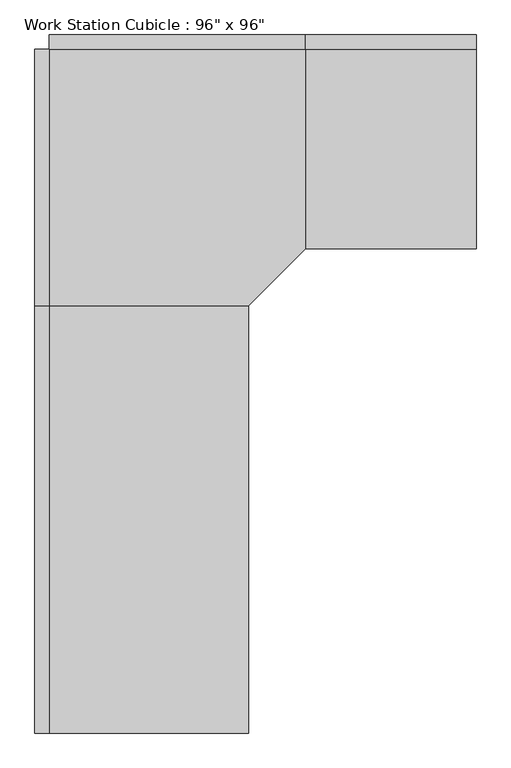
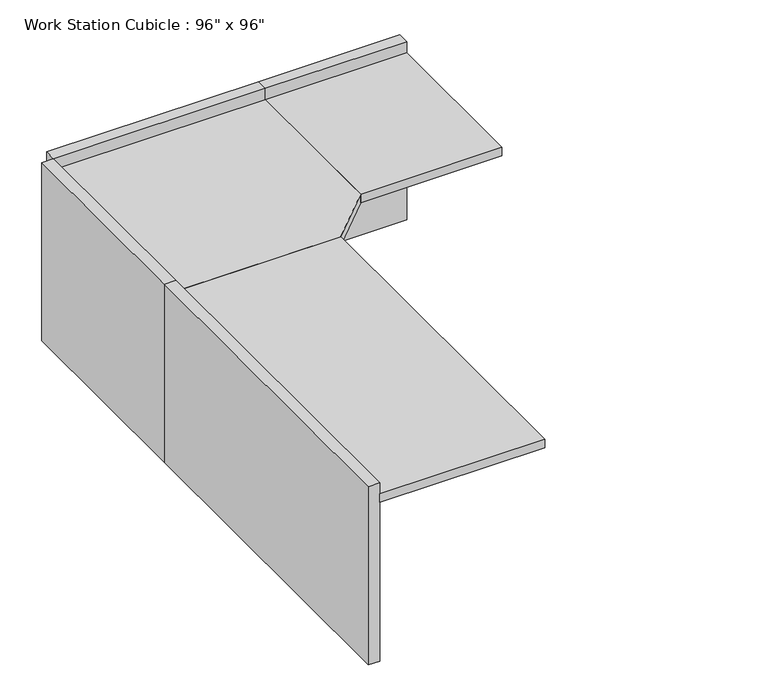
"""IFC4 building model written with IfcOpenShell, lengths in millimetres: furniture geometry."""

from ifc_helpers import new_model, si_unit, frame, origin, origin_with_axes, place, context, project, spatial, polyline, outline, extrude, source, transform, mapped, element, save


def furniture_4f21b5ed(model_context):
    return source(origin(), model_context, "Body", "SweptSolid", [
        extrude(outline(polyline([(-80.9317522, -545.8230076), (833.4682478, -545.8230076), (833.4682478, -1257.0230076), (630.2682478, -1460.2230076), (-80.9317522, -1460.2230076), (-80.9317522, -545.8230076)])), frame((0.0, 0.0, 723.9), z_axis=(0.0, 0.0, 1.0), x_axis=(1.0, 0.0, 0.0)), (0.0, 0.0, 1.0), 38.1),
        extrude(outline(polyline([(630.2682478, -2984.2230076), (-80.9317522, -2984.2230076), (-80.9317522, -1460.2230076), (630.2682478, -1460.2230076), (630.2682478, -2984.2230076)])), frame((0.0, 0.0, 723.9), z_axis=(0.0, 0.0, 1.0), x_axis=(1.0, 0.0, 0.0)), (0.0, 0.0, 1.0), 38.1),
        extrude(outline(polyline([(1443.0682478, -1257.0230076), (833.4682478, -1257.0230076), (833.4682478, -545.8230076), (1443.0682478, -545.8230076), (1443.0682478, -1257.0230076)])), frame((0.0, 0.0, 723.9), z_axis=(0.0, 0.0, 1.0), x_axis=(1.0, 0.0, 0.0)), (0.0, 0.0, 1.0), 38.1),
        extrude(outline(polyline([(1443.0682478, -545.8230076), (833.4682478, -545.8230076), (833.4682478, -495.0230076), (1443.0682478, -495.0230076), (1443.0682478, -545.8230076)])), origin_with_axes(), (0.0, 0.0, 1.0), 812.8),
        extrude(outline(polyline([(833.4682478, -545.8230076), (-80.9317522, -545.8230076), (-80.9317522, -495.0230076), (833.4682478, -495.0230076), (833.4682478, -545.8230076)])), origin_with_axes(), (0.0, 0.0, 1.0), 812.8),
        extrude(outline(polyline([(-80.9317522, -1460.2230076), (-131.7317522, -1460.2230076), (-131.7317522, -545.8230076), (-80.9317522, -545.8230076), (-80.9317522, -1460.2230076)])), origin_with_axes(), (0.0, 0.0, 1.0), 812.8),
        extrude(outline(polyline([(-80.9317522, -2984.2230076), (-131.7317522, -2984.2230076), (-131.7317522, -1460.2230076), (-80.9317522, -1460.2230076), (-80.9317522, -2984.2230076)])), origin_with_axes(), (0.0, 0.0, 1.0), 812.8),
    ])


if __name__ == "__main__":
    model = new_model("IFC4")
    model_context = context("Model", 3, world=origin())
    ifc_project = project(units=[si_unit("LENGTHUNIT", "METRE", prefix="MILLI")], contexts=[model_context])
    site = spatial("IfcSite", under=ifc_project)
    building = spatial("IfcBuilding", under=site)
    placement = place(None, origin())
    furniture_shape = furniture_4f21b5ed(model_context)
    element("IfcFurniture", 1, ObjectType="Work Station Cubicle : 96\" x 96\"", at=placement, inside=building, context=model_context, shape_type="MappedRepresentation", body=[
        mapped(furniture_shape, transform((0.0, 0.0, 0.0), x_axis=(1.0, 0.0, 0.0), y_axis=(0.0, 1.0, 0.0), z_axis=(0.0, 0.0, 1.0))),
    ])
    save(model, "model.ifc")

# Revit data of these elements
# Type "Work Station Cubicle : 96\" x 96\""
#   Assembly Code = "E2020"
#   Desktop Height = 2' - 6"
#   Desktop1 Width = 2' - 4"
#   Desktop2 Width = 2' - 4"
#   Panel Height = 2' - 8"
#   Panel1 Length = 5' - 0"
#   Panel2 Length = 2' - 0"
#   Cube Panel Material = Textile - Light Gray
#   Work Top Material = Laminate, Ivory, Matte
#   Default Elevation = 0
# Element 1 (IfcFurniture, "Work Station Cubicle : 96\" x 96\"")
#   Materials on its faces: "Textile - Light Gray", "Laminate, Ivory, Matte"
# Materials
#   "Textile - Light Gray": class "Fabric", colour RGB 204 204 204, transparency 0
#   "Laminate, Ivory, Matte": class "Plastic", colour RGB 247 247 239, transparency 0, Description = "Plastic Laminate - Ivory, Matte", Cost = 0
